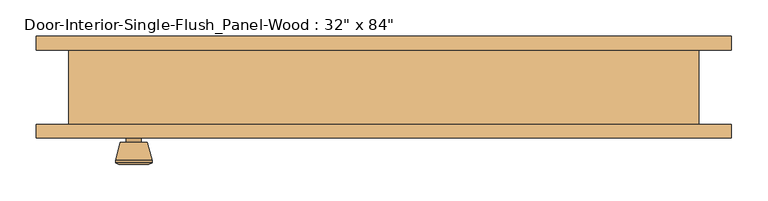
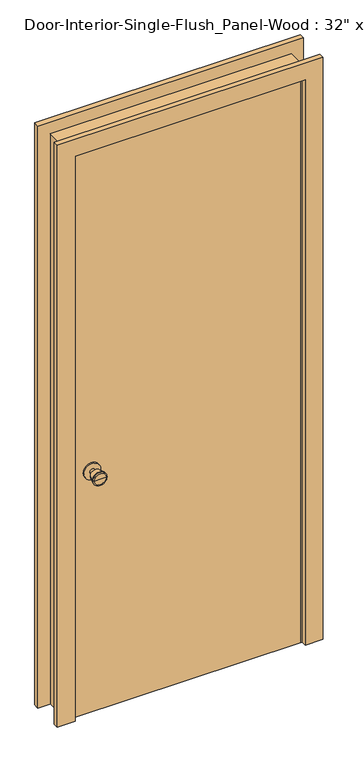
"""IFC4 building model written with IfcOpenShell, lengths in millimetres: door geometry."""

from ifc_helpers import new_model, si_unit, point, frame, frame_2d, origin, origin_with_axes, place, context, project, spatial, polyline, circle_curve, trimmed, segment, composite_curve, outline, extrude, faceted_brep, source, transform, mapped, element, save
from ifc_brep_helpers import plane_surface, cylinder_surface, revolved_surface, advanced_brep


def door_3c591639(model_context):
    return source(origin(), model_context, "Body", "SolidModel", [
        advanced_brep(
        [(-342.9, -6.7, 914.4), (-352.9, -6.7, 914.4), (-332.9, -6.7, 914.4), (-322.4241324, 42.3, 914.4), (-363.3758676, 42.3, 914.4), (-342.9, 42.3, 914.4), (-317.9, 40.4721319, 914.4), (-367.9, 40.4721319, 914.4), (-317.9, 37.0084537, 914.4), (-367.9, 37.0084537, 914.4), (-324.263764, 12.3, 914.4), (-361.536236, 12.3, 914.4), (-332.9, 12.3, 914.4), (-352.9, 12.3, 914.4)],
        [
            (0, 1),
            (1, 2, circle_curve(frame((-342.9, -6.7, 914.4), z_axis=(0.0, -1.0, 0.0), x_axis=(-1.0, 0.0, 0.0)), 10.0)),
            (2, 0),
            (2, 1, circle_curve(frame((-342.9, -6.7, 914.4), z_axis=(0.0, -1.0, 0.0), x_axis=(-1.0, 0.0, 0.0)), 10.0)),
            (3, 4, circle_curve(frame((-342.9, 42.3, 914.4), z_axis=(0.0, 1.0, 0.0), x_axis=(-1.0, 0.0, 0.0)), 20.4758676)),
            (4, 5),
            (5, 3),
            (4, 3, circle_curve(frame((-342.9, 42.3, 914.4), z_axis=(0.0, 1.0, 0.0), x_axis=(-1.0, 0.0, 0.0)), 20.4758676)),
            (6, 7, circle_curve(frame((-342.9, 40.4721319, 914.4), z_axis=(0.0, 1.0, 0.0), x_axis=(-1.0, 0.0, 0.0)), 25.0)),
            (7, 4),
            (3, 6),
            (7, 6, circle_curve(frame((-342.9, 40.4721319, 914.4), z_axis=(0.0, 1.0, 0.0), x_axis=(-1.0, 0.0, 0.0)), 25.0)),
            (8, 9, circle_curve(frame((-342.9, 37.0084537, 914.4), z_axis=(0.0, 1.0, 0.0), x_axis=(-1.0, 0.0, 0.0)), 25.0)),
            (9, 7),
            (6, 8),
            (9, 8, circle_curve(frame((-342.9, 37.0084537, 914.4), z_axis=(0.0, 1.0, 0.0), x_axis=(-1.0, 0.0, 0.0)), 25.0)),
            (10, 11, circle_curve(frame((-342.9, 12.3, 914.4), z_axis=(0.0, 1.0, 0.0), x_axis=(-1.0, 0.0, 0.0)), 18.636236)),
            (11, 9),
            (8, 10),
            (11, 10, circle_curve(frame((-342.9, 12.3, 914.4), z_axis=(0.0, 1.0, 0.0), x_axis=(-1.0, 0.0, 0.0)), 18.636236)),
            (12, 13, circle_curve(frame((-342.9, 12.3, 914.4), z_axis=(0.0, 1.0, 0.0), x_axis=(-1.0, 0.0, 0.0)), 10.0)),
            (13, 11),
            (10, 12),
            (13, 12, circle_curve(frame((-342.9, 12.3, 914.4), z_axis=(0.0, 1.0, 0.0), x_axis=(-1.0, 0.0, 0.0)), 10.0)),
            (1, 13),
            (12, 2),
        ],
        [
            plane_surface(frame((-342.9, -6.7, 914.4), z_axis=(0.0, -1.0, 0.0), x_axis=(-1.0, 0.0, 0.0))),
            plane_surface(frame((-342.9, 42.3, 914.4), z_axis=(0.0, 1.0, 0.0), x_axis=(-1.0, 0.0, 0.0))),
            revolved_surface(polyline([(-363.3758676, 42.3, 914.4), (-367.9, 40.4721319, 914.4)]), (-342.9, -6.7, 914.4), (0.0, -1.0, 0.0)),
            cylinder_surface(frame((-342.9, -6.7, 914.4), z_axis=(0.0, -1.0, 0.0), x_axis=(-1.0, 0.0, 0.0)), 25.0),
            revolved_surface(polyline([(-367.9, 37.0084537, 914.4), (-361.536236, 12.3, 914.4)]), (-342.9, -6.7, 914.4), (0.0, -1.0, 0.0)),
            plane_surface(frame((-342.9, 12.3, 914.4), z_axis=(0.0, -1.0, 0.0), x_axis=(-1.0, 0.0, 0.0))),
            cylinder_surface(frame((-342.9, -6.7, 914.4), z_axis=(0.0, -1.0, 0.0), x_axis=(-1.0, 0.0, 0.0)), 10.0),
        ],
        [
            (0, [[1, 2, 3]]),
            (0, [[-3, 4, -1]]),
            (1, [[5, 6, 7]]),
            (1, [[8, -7, -6]]),
            (2, [[9, 10, -5, 11]]),
            (2, [[12, -11, -8, -10]]),
            (3, [[13, 14, -9, 15]]),
            (3, [[16, -15, -12, -14]]),
            (4, [[17, 18, -13, 19]]),
            (4, [[20, -19, -16, -18]]),
            (5, [[21, 22, -17, 23]]),
            (5, [[24, -23, -20, -22]]),
            (6, [[-2, 25, -21, 26]]),
            (6, [[-4, -26, -24, -25]]),
        ],
    ),
        extrude(outline(composite_curve([segment(trimmed(circle_curve(frame_2d((914.4, -342.9)), 30.0), [point((914.4, -372.9))], [point((914.4, -312.9))], False, "CARTESIAN"), True, "CONTINUOUS"), segment(trimmed(circle_curve(frame_2d((914.4, -342.9)), 30.0), [point((914.4, -312.9))], [point((914.4, -372.9))], False, "CARTESIAN"), True, "CONTINUOUS")], self_intersect=False)), frame((0.0, -12.7, 0.0), z_axis=(0.0, 1.0, 0.0), x_axis=(0.0, 0.0, 1.0)), (0.0, 0.0, 1.0), 6.0),
        advanced_brep(
        [(-342.9, -53.625, 914.4), (-332.9, -53.625, 914.4), (-352.9, -53.625, 914.4), (-322.4241324, -102.625, 914.4), (-342.9, -102.625, 914.4), (-363.3758676, -102.625, 914.4), (-317.9, -100.7971319, 914.4), (-367.9, -100.7971319, 914.4), (-317.9, -97.3334537, 914.4), (-367.9, -97.3334537, 914.4), (-324.263764, -72.625, 914.4), (-361.536236, -72.625, 914.4), (-332.9, -72.625, 914.4), (-352.9, -72.625, 914.4)],
        [
            (0, 1),
            (1, 2, circle_curve(frame((-342.9, -53.625, 914.4), z_axis=(0.0, 1.0, 0.0), x_axis=(-1.0, 0.0, 0.0)), 10.0)),
            (2, 0),
            (2, 1, circle_curve(frame((-342.9, -53.625, 914.4), z_axis=(0.0, 1.0, 0.0), x_axis=(-1.0, 0.0, 0.0)), 10.0)),
            (3, 4),
            (4, 5),
            (5, 3, circle_curve(frame((-342.9, -102.625, 914.4), z_axis=(0.0, -1.0, 0.0), x_axis=(-1.0, 0.0, 0.0)), 20.4758676)),
            (3, 5, circle_curve(frame((-342.9, -102.625, 914.4), z_axis=(0.0, -1.0, 0.0), x_axis=(-1.0, 0.0, 0.0)), 20.4758676)),
            (6, 3),
            (5, 7),
            (7, 6, circle_curve(frame((-342.9, -100.7971319, 914.4), z_axis=(0.0, -1.0, 0.0), x_axis=(-1.0, 0.0, 0.0)), 25.0)),
            (6, 7, circle_curve(frame((-342.9, -100.7971319, 914.4), z_axis=(0.0, -1.0, 0.0), x_axis=(-1.0, 0.0, 0.0)), 25.0)),
            (8, 6),
            (7, 9),
            (9, 8, circle_curve(frame((-342.9, -97.3334537, 914.4), z_axis=(0.0, -1.0, 0.0), x_axis=(-1.0, 0.0, 0.0)), 25.0)),
            (8, 9, circle_curve(frame((-342.9, -97.3334537, 914.4), z_axis=(0.0, -1.0, 0.0), x_axis=(-1.0, 0.0, 0.0)), 25.0)),
            (10, 8),
            (9, 11),
            (11, 10, circle_curve(frame((-342.9, -72.625, 914.4), z_axis=(0.0, -1.0, 0.0), x_axis=(-1.0, 0.0, 0.0)), 18.636236)),
            (10, 11, circle_curve(frame((-342.9, -72.625, 914.4), z_axis=(0.0, -1.0, 0.0), x_axis=(-1.0, 0.0, 0.0)), 18.636236)),
            (12, 10),
            (11, 13),
            (13, 12, circle_curve(frame((-342.9, -72.625, 914.4), z_axis=(0.0, -1.0, 0.0), x_axis=(-1.0, 0.0, 0.0)), 10.0)),
            (12, 13, circle_curve(frame((-342.9, -72.625, 914.4), z_axis=(0.0, -1.0, 0.0), x_axis=(-1.0, 0.0, 0.0)), 10.0)),
            (1, 12),
            (13, 2),
        ],
        [
            plane_surface(frame((-342.9, -53.625, 914.4), z_axis=(0.0, 1.0, 0.0), x_axis=(-1.0, 0.0, 0.0))),
            plane_surface(frame((-342.9, -102.625, 914.4), z_axis=(0.0, -1.0, 0.0), x_axis=(-1.0, 0.0, 0.0))),
            revolved_surface(polyline([(-363.3758676, -102.625, 914.4), (-367.9, -100.7971319, 914.4)]), (-342.9, -53.625, 914.4), (0.0, 1.0, 0.0)),
            cylinder_surface(frame((-342.9, -53.625, 914.4), z_axis=(0.0, 1.0, 0.0), x_axis=(-1.0, 0.0, 0.0)), 25.0),
            revolved_surface(polyline([(-367.9, -97.3334537, 914.4), (-361.536236, -72.625, 914.4)]), (-342.9, -53.625, 914.4), (0.0, 1.0, 0.0)),
            plane_surface(frame((-342.9, -72.625, 914.4), z_axis=(0.0, 1.0, 0.0), x_axis=(-1.0, 0.0, 0.0))),
            cylinder_surface(frame((-342.9, -53.625, 914.4), z_axis=(0.0, 1.0, 0.0), x_axis=(-1.0, 0.0, 0.0)), 10.0),
        ],
        [
            (0, [[1, 2, 3]]),
            (0, [[-3, 4, -1]]),
            (1, [[5, 6, 7]]),
            (1, [[-6, -5, 8]]),
            (2, [[9, -7, 10, 11]]),
            (2, [[-10, -8, -9, 12]]),
            (3, [[13, -11, 14, 15]]),
            (3, [[-14, -12, -13, 16]]),
            (4, [[17, -15, 18, 19]]),
            (4, [[-18, -16, -17, 20]]),
            (5, [[21, -19, 22, 23]]),
            (5, [[-22, -20, -21, 24]]),
            (6, [[25, -23, 26, -2]]),
            (6, [[-26, -24, -25, -4]]),
        ],
    ),
        extrude(outline(composite_curve([segment(trimmed(circle_curve(frame_2d((914.4, -342.9)), 30.0), [point((914.4, -372.9))], [point((914.4, -312.9))], False, "CARTESIAN"), True, "CONTINUOUS"), segment(trimmed(circle_curve(frame_2d((914.4, -342.9)), 30.0), [point((914.4, -312.9))], [point((914.4, -372.9))], False, "CARTESIAN"), True, "CONTINUOUS")], self_intersect=False)), frame((0.0, -53.625, 0.0), z_axis=(0.0, 1.0, 0.0), x_axis=(0.0, 0.0, 1.0)), (0.0, 0.0, 1.0), 6.0),
        extrude(outline(polyline([(406.4, -12.7), (406.4, -47.625), (-406.4, -47.625), (-406.4, -12.7), (406.4, -12.7)])), origin_with_axes(), (0.0, 0.0, 1.0), 2133.6),
        faceted_brep([(431.8, -47.625, 0.0), (406.4, -47.625, 0.0), (406.4, -12.7, 0.0), (393.7, -12.7, 0.0), (393.7, 22.225, 0.0), (406.4, 22.225, 0.0), (406.4, 53.975, 0.0), (431.8, 53.975, 0.0), (431.8, 53.975, 2159.0), (431.8, -47.625, 2159.0), (406.4, 53.975, 2133.6), (-406.4, 53.975, 2133.6), (-406.4, 53.975, 0.0), (-431.8, 53.975, 0.0), (-431.8, 53.975, 2159.0), (406.4, 22.225, 2133.6), (393.7, 22.225, 2120.9), (-393.7, 22.225, 2120.9), (-393.7, 22.225, 0.0), (-406.4, 22.225, 0.0), (-406.4, 22.225, 2133.6), (393.7, -12.7, 2120.9), (406.4, -12.7, 2133.6), (-406.4, -12.7, 2133.6), (-406.4, -12.7, 0.0), (-393.7, -12.7, 0.0), (-393.7, -12.7, 2120.9), (406.4, -47.625, 2133.6), (-431.8, -47.625, 2159.0), (-431.8, -47.625, 0.0), (-406.4, -47.625, 0.0), (-406.4, -47.625, 2133.6)], [[[0, 1, 2, 3, 4, 5, 6, 7]], [[7, 8, 9, 0]], [[6, 10, 11, 12, 13, 14, 8, 7]], [[5, 15, 10, 6]], [[4, 16, 17, 18, 19, 20, 15, 5]], [[3, 21, 16, 4]], [[2, 22, 23, 24, 25, 26, 21, 3]], [[1, 27, 22, 2]], [[0, 9, 28, 29, 30, 31, 27, 1]], [[8, 14, 28, 9]], [[15, 20, 11, 10]], [[21, 26, 17, 16]], [[27, 31, 23, 22]], [[29, 13, 12, 19, 18, 25, 24, 30]], [[14, 13, 29, 28]], [[20, 19, 12, 11]], [[26, 25, 18, 17]], [[31, 30, 24, 23]]]),
        extrude(outline(polyline([(0.0, 476.25), (2203.45, 476.25), (2203.45, -476.25), (0.0, -476.25), (0.0, -412.75), (2139.95, -412.75), (2139.95, 412.75), (0.0, 412.75), (0.0, 476.25)])), frame((0.0, 53.975, 0.0), z_axis=(0.0, 1.0, 0.0), x_axis=(0.0, 0.0, 1.0)), (0.0, 0.0, 1.0), 19.05),
        extrude(outline(polyline([(0.0, 476.25), (2203.45, 476.25), (2203.45, -476.25), (0.0, -476.25), (0.0, -412.75), (2139.95, -412.75), (2139.95, 412.75), (0.0, 412.75), (0.0, 476.25)])), frame((0.0, -66.675, 0.0), z_axis=(0.0, 1.0, 0.0), x_axis=(0.0, 0.0, 1.0)), (0.0, 0.0, 1.0), 19.05),
    ])


if __name__ == "__main__":
    model = new_model("IFC4")
    model_context = context("Model", 3, world=origin())
    ifc_project = project(units=[si_unit("LENGTHUNIT", "METRE", prefix="MILLI")], contexts=[model_context])
    site = spatial("IfcSite", under=ifc_project)
    building = spatial("IfcBuilding", under=site)
    placement = place(None, origin())
    door_shape = door_3c591639(model_context)
    element("IfcDoor", 1, ObjectType="Door-Interior-Single-Flush_Panel-Wood : 32\" x 84\"", at=placement, inside=building, context=model_context, shape_type="MappedRepresentation", body=[
        mapped(door_shape, transform((0.0, 0.0, 0.0), x_axis=(1.0, 0.0, 0.0), y_axis=(0.0, 1.0, 0.0), z_axis=(0.0, 0.0, 1.0))),
    ])
    save(model, "model.ifc")

# Revit data of these elements
# Type "Door-Interior-Single-Flush_Panel-Wood : 32\" x 84\""
#   Type Mark = "11"
#   Assembly Code = "C1020300"
#   Analytic Construction = "Wooden"
#   Thickness = 0' - 1 3/8"
#   Thermal Resistance (R) = 2.5876 (h·ft²·°F)/BTU
#   Swing Angle [instance default] = 90.00°
#   Rough Width = 2' - 10"
#   Rough Height = 7' - 1"
#   Height = 7' - 0"
#   Width = 2' - 8"
#   Heat Transfer Coefficient (U) = 0.3865 BTU/(h·ft²·°F)
#   Trim Material = Cherry
#   Panel Material = Cherry
#   Frame Material = Cherry
#   Door Handle Material = Aluminum
#   Visual Light Transmittance = 0
#   Solar Heat Gain Coefficient = 0
#   Wall Closure = (empty or 0)
#   Function = (empty or 0)
# Element 1 (IfcDoor, "Door-Interior-Single-Flush_Panel-Wood : 32\" x 84\"")
#   Materials on its faces: "Cherry", "Aluminum"
# Materials
#   "Cherry": class "Wood", colour RGB 226 177 128, transparency 0, Description = "Prunus Serotina", Cost = 0
#   "Aluminum": class "Metal", colour RGB 247 247 247, transparency 0, Description = "Aluminum 6061", Cost = 0
